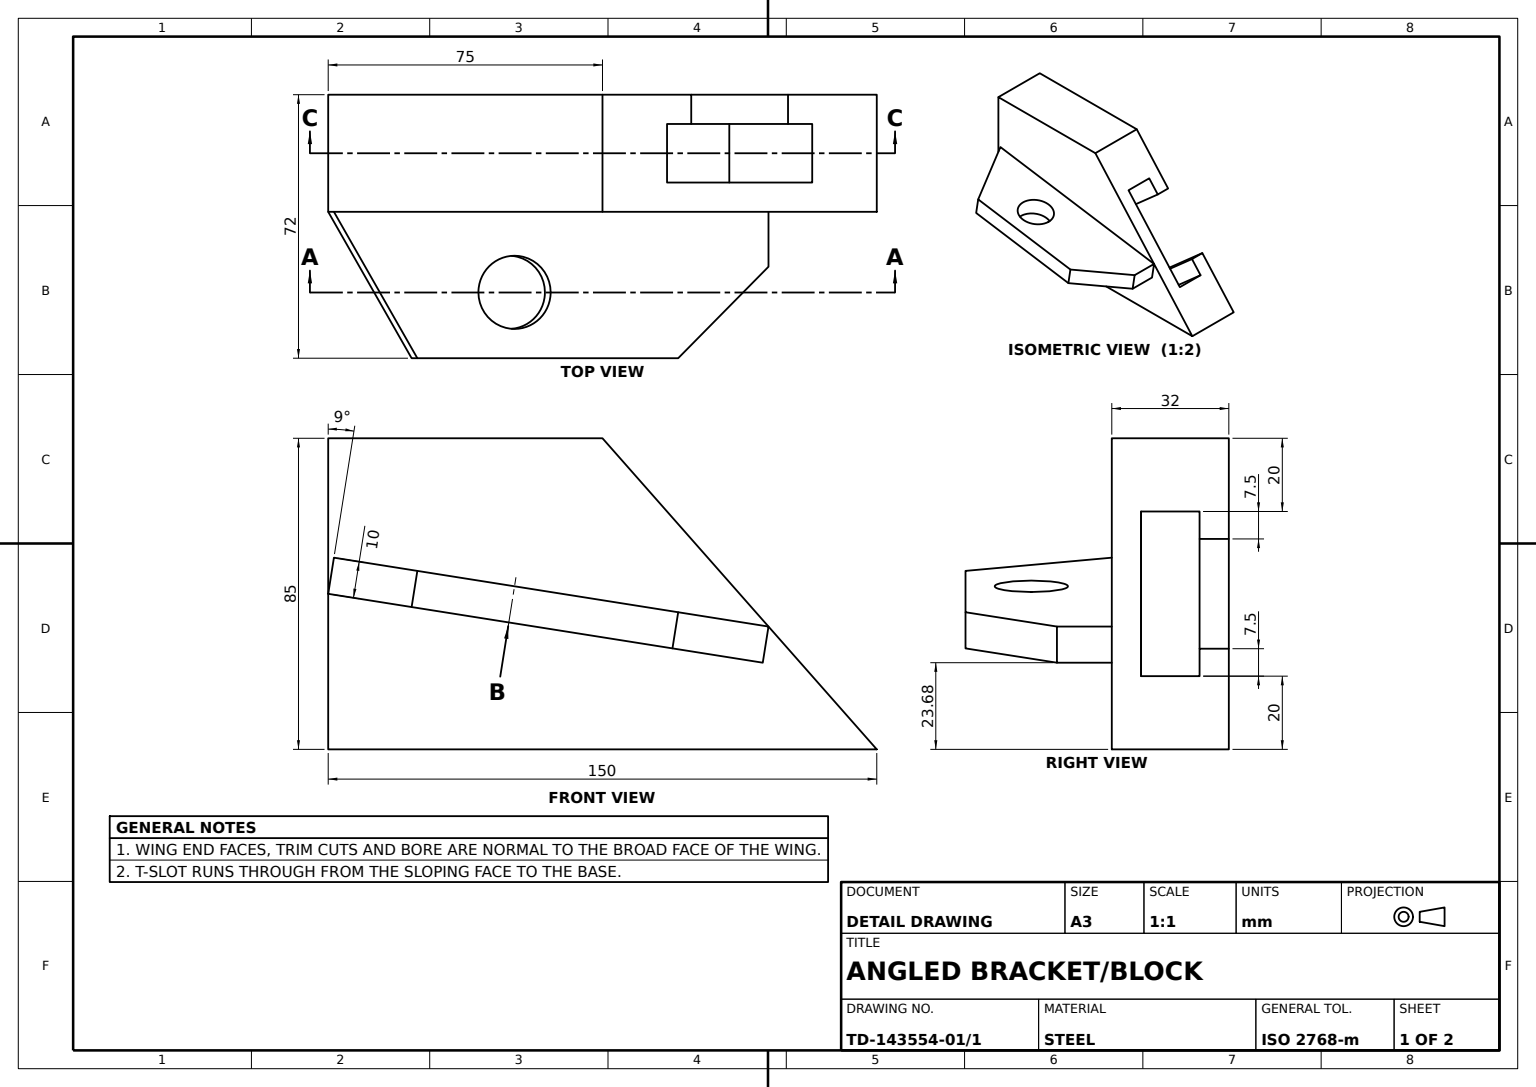
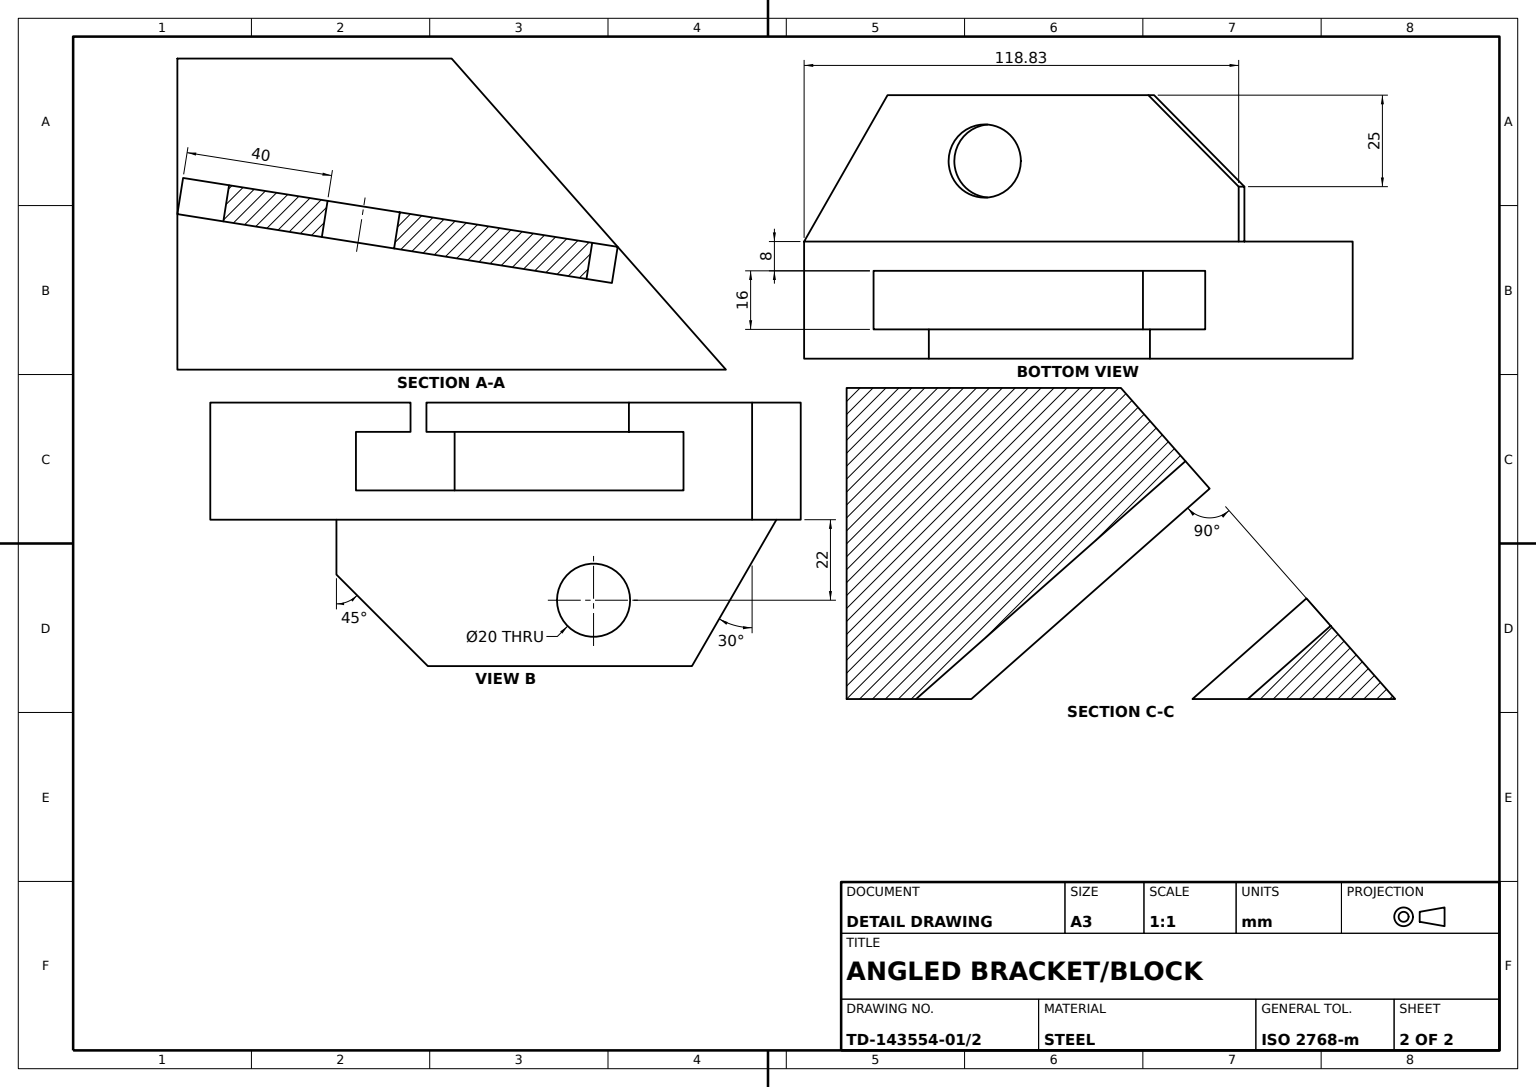
SolidWorks part; units mm, degrees
material "Plain Carbon Steel"
ref_plane "Front Plane" through (0, 0, 0) normal (0, 0, 1) x (1, 0, 0)
ref_plane "Top Plane" through (0, 0, 0) normal (0, 1, 0) x (1, 0, 0)
ref_plane "Right Plane" through (0, 0, 0) normal (1, 0, 0) x (0, 0, -1)
sketch "Base Block Sketch" plane through (0, 0, 0) normal (0, 0, 1) x (1, 0, 0)
  line L0 (75, 85) -> (150, 0)
  line L1 (0, 0) -> (150, 0)
  line L2 (0, 0) -> (0, 85)
  line L3 (0, 85) -> (75, 85)
  dimension "D1" = 150
  dimension "D2" = 85
  dimension "D3" = 75
extrude "Base Block" add sketch "Base Block Sketch" against normal blind 32
sketch "Slot Cut Sketch" plane through (84.3385, 74.4163, 0) normal (0.7498, 0.6616, 0) x (0, 0, -1)
  line L0 (16, 14.1146) -> (16, -99.2432) construction
  line L5 (32, 14.1146) -> (0, 14.1146) construction
  line L6 (32, -99.2432) -> (0, -99.2432) construction
  line L7 (0, -42.5643) -> (32, -42.5643) construction
  line L9 (32, -99.2432) -> (32, 14.1146) construction
  line L10 (24, -22.5643) -> (32, -22.5643)
  line L11 (8, -72.5643) -> (24, -72.5643)
  line L12 (8, -72.5643) -> (8, -12.5643)
  line L13 (8, -12.5643) -> (24, -12.5643)
  line L14 (24, -72.5643) -> (24, -62.5643)
  line L15 (24, -22.5643) -> (24, -12.5643)
  line L16 (32, -22.5643) -> (32, -62.5643)
  line L17 (24, -62.5643) -> (32, -62.5643)
  point P0 (16, -42.5643)
  dimension "D1" = 60
  dimension "D2" = 16
  dimension "D3" = 40
  dimension "D4" = 20
  dimension "D5" = 8
  dimension "D6" = 26.6789
extrude "Slot Cut" cut sketch "Slot Cut Sketch" against normal blind 140
sketch "Angled Wing Sketch" plane through (0, 0, 0) normal (0, 0, 1) x (1, 0, 0)
  line L0 (0, 42.5) -> (118.8269, 23.6797)
  line L1 (0, 85) -> (0, 0) construction
  line L2 (1.5643, 52.3769) -> (120.3913, 33.5565)
  line L3 (75, 85) -> (0, 85) construction
  line L4 (1.5643, 52.3769) -> (136.4567, 31.012) construction
  line L5 (0, 42.5) -> (1.5643, 52.3769)
  line L6 (0, 42.5) -> (134.8923, 21.1352) construction
  line L8 (120.3913, 33.5565) -> (118.8269, 23.6797)
  line L9 (1.5643, 52.3769) -> (120.3913, 33.5565)
  line L10 (118.8269, 23.6797) -> (0, 42.5)
  dimension "D2" = 9
  dimension "D3" = 118.8269
  dimension "D1" = 10
extrude "Angled Wing" add sketch "Angled Wing Sketch" along normal blind 40 contours L8 L2 L5 L0
sketch "Wing Trim Cut Sketch" plane through (8.131, 51.3368, 0) normal (0.1564, 0.9877, 0) x (0.9877, -0.1564, 0)
  line L0 (-6.6485, 0) -> (20.1725, -46.4553)
  line L1 (113.6597, -15) -> (81.4808, -47.1789)
  line L2 (113.6597, -40) -> (113.6597, 0) construction
  line L3 (60.7797, 0) -> (-13.2969, 0) construction
  line L4 (-6.6485, -40) -> (-6.6485, 0) construction
  line L5 (-6.6485, -40) -> (113.6597, -40) construction
  line L6 (-6.6485, 0) -> (-6.6485, -46.4553)
  line L7 (-6.6485, -46.4553) -> (20.1725, -46.4553)
  line L8 (81.4808, -47.1789) -> (138.0763, -47.1789)
  line L9 (138.0763, -47.1789) -> (113.6597, -15)
  circle A0 centre (43.3515, -22) radius 10
  dimension "D6" = 20
  dimension "D1" = 22
  dimension "D2" = 30
  dimension "D3" = 45
  dimension "D4" = 25
  dimension "D5" = 50
  dimension "D7" = 26.821
  dimension "D8" = 88.1293
  dimension "D9" = 144.7247
extrude "Wing Trim Cut" cut sketch "Wing Trim Cut Sketch" against normal blind 40
